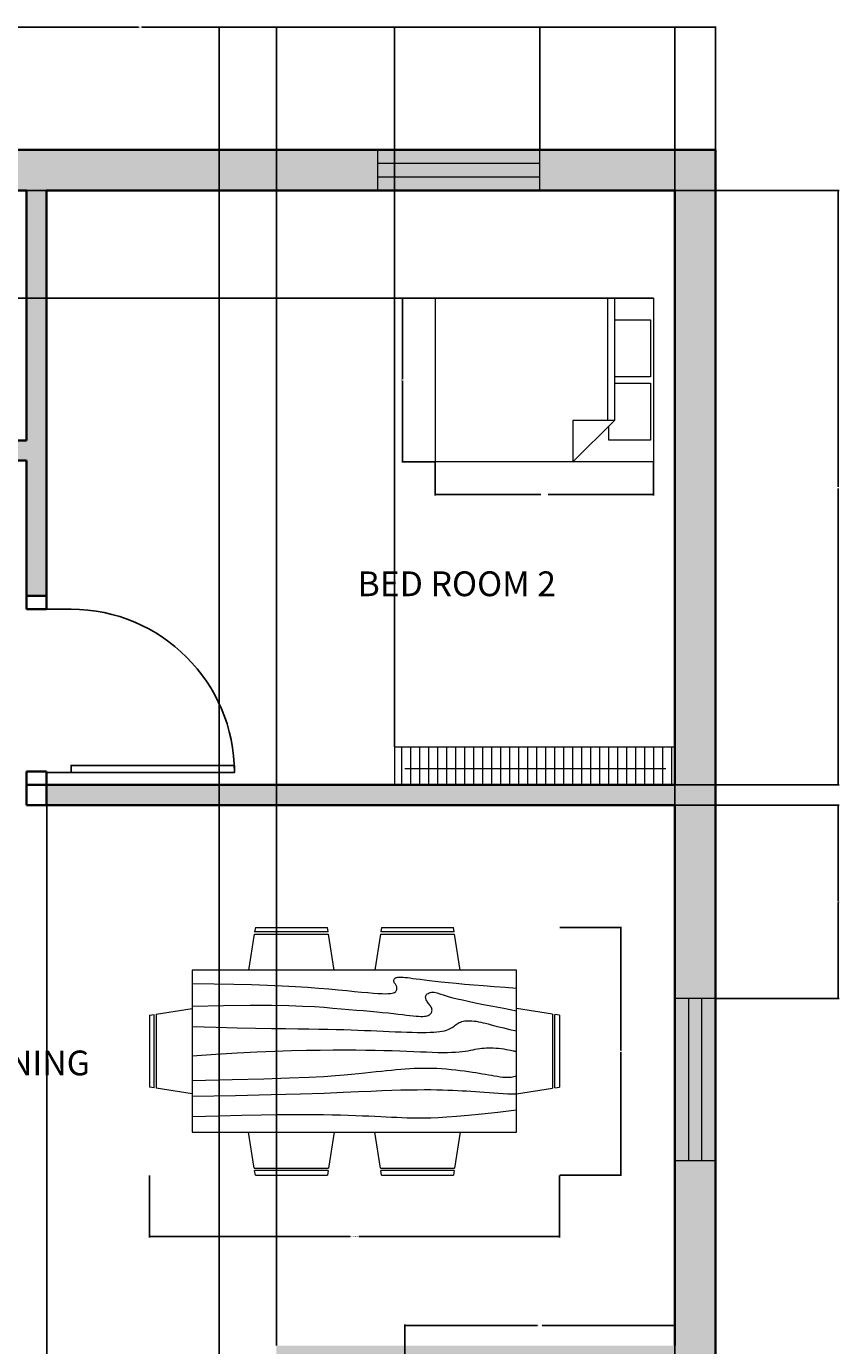
# Model space of a CAD drawing. Units: inches. Extents: x 1839 to 2285, y 722 to 1311.
# Tile 7 of 7: x 2105 to 2285, y 1018 to 1311. Entities that reach past the tile are written whole.
import ezdxf

# ---------------------------------------------------------------- set-up
doc = ezdxf.new("R2010")
doc.units = ezdxf.units.IN
for name, color, linetype, lineweight in [('A-ANNO-DIMS', 2, 'Continuous', 18), ('A-AREA-IDEN', 7, 'Continuous', 18), ('A-DOOR', 3, 'Continuous', 25), ('A-FLOR-CASE', 8, 'Continuous', 18), ('A-FLOR-PATT', 8, 'Continuous', 13), ('A-FURN', 8, 'Continuous', 18), ('A-GLAZ', 4, 'Continuous', 18), ('A-GLAZ-PATT', 9, 'Continuous', 13), ('A-WALL', 7, 'Continuous', 35)]:
    doc.layers.add(name, color=color, linetype=linetype, lineweight=lineweight)
doc.layers.add('A-WALL-PATT', color=18, linetype='Continuous', lineweight=13, true_color=0x000000)
doc.styles.get("Standard").update_dxf_attribs({"font": 'arial.ttf'})
doc.dimstyles.get("Standard").update_dxf_attribs({"dimtxt": 0.18, "dimasz": 0.18, "dimexe": 0.18, "dimexo": 0.0625, "dimgap": 0.09, "dimtad": 0, "dimtih": 1, "dimtoh": 1, "dimdec": 4, "dimzin": 0, "dimdsep": 46, "dimtxsty": 'Standard', "dimcen": 0.09, "dimadec": 0, "dimazin": 0, "dimtfac": 1, "dimtdec": 4, "dimtofl": 0, "dimtmove": 0, "dimatfit": 3, "dimfxl": 1, "dimtolj": 1, "dimtzin": 0, "dimarcsym": 0})

# ---------------------------------------------------------------- blocks, each defined once
blk = doc.blocks.new('*U3')
for p, q in [((0, 0), (0, -6)), ((-40, 0), (-40, -6))]:
    blk.add_line(p, q)
blk.add_lwpolyline([(0, 0), (0, 40), (-1.75, 40), (-1.75, 0)], close=True)
blk.add_arc((0, 0), 40, 90, 180)
blk = doc.blocks.new('Bed - Queen')
for p, q in [((0, -80.00003), (0, 0)), ((0, 0), (59.99999, 0)), ((59.99999, 0), (59.99999, -80.00003)), ((7.99999, -1.2), (28.79998, -1.2)), ((7.99999, -14.4), (7.99999, -1.2)), ((28.79998, -1.2), (28.79998, -14.4)), ((31.19999, -1.2), (51.99999, -1.2)), ((31.19999, -14.4), (31.19999, -1.2)), ((51.99999, -1.2), (51.99999, -16.4)), ((0, -14.4), (44.8, -14.4)), ((59.99999, -29.6), (44.8, -14.4)), ((44.8, -14.4), (44.8, -29.6)), ((44.8, -16.8), (0, -16.8)), ((51.99999, -16.4), (46.79936, -16.4)), ((44.8, -29.6), (59.99999, -29.6)), ((59.99999, -80.00003), (0, -80.00003))]:
    blk.add_line(p, q)
blk = doc.blocks.new('Dining Set - 36 x 72 in.')
for p, q in [((-22, 27.5), (-22.1562, 26.50042)), ((-5.8416, 26.5), (-22.1534, 26.5)), ((-22, 27.5), (-6, 27.5)), ((-5.8437, 26.49966), (-6, 27.5)), ((6, 27.5), (5.8438, 26.50042)), ((22.1584, 26.5), (5.8466, 26.5)), ((6, 27.5), (22, 27.5)), ((22.1563, 26.49966), (22, 27.5)), ((-22.2343, 26.00059), (-23.4847, 17.99762)), ((-22.2304, 26), (-5.7608, 26)), ((-4.5152, 17.99762), (-5.7655, 25.99926)), ((5.7657, 26.00059), (4.5153, 17.99762)), ((5.7696, 26), (22.2392, 26)), ((23.4848, 17.99762), (22.2345, 25.99926)), ((36, 18), (-36, 18)), ((-36, 18), (-36, -18)), ((36, -18), (36, 18)), ((-44.0006, 8.23428), (-35.9976, 9.48474)), ((44.0006, 8.23428), (35.9976, 9.48474)), ((-45.5, 8), (-44.5004, 8.15617)), ((-45.5, 8), (-45.5, -8)), ((-44.5, -8.15843), (-44.5, 8.15338)), ((-44, 8.23041), (-44, -8.23915)), ((44, 8.23041), (44, -8.23915)), ((44.5, -8.15843), (44.5, 8.15338)), ((45.5, 8), (44.5005, 8.15617)), ((45.5, 8), (45.5, -8)), ((-44.4997, -8.15631), (-45.5, -8)), ((-35.9976, -9.48476), (-43.9993, -8.2345)), ((35.9976, -9.48476), (43.9993, -8.2345)), ((44.4997, -8.15631), (45.5, -8)), ((-36, -18), (36, -18)), ((-22.2343, -26.0006), (-23.4847, -17.99762)), ((-4.5152, -17.99762), (-5.7655, -25.99928)), ((5.7657, -26.0006), (4.5153, -17.99762)), ((23.4848, -17.99762), (22.2345, -25.99928)), ((-22.2304, -26), (-5.7608, -26)), ((5.7696, -26), (22.2392, -26)), ((-22, -27.5), (-22.1562, -26.50044)), ((-5.8416, -26.5), (-22.1534, -26.5)), ((-22, -27.5), (-6, -27.5)), ((-5.8437, -26.49967), (-6, -27.5)), ((6, -27.5), (5.8438, -26.50044)), ((22.1584, -26.5), (5.8466, -26.5)), ((6, -27.5), (22, -27.5)), ((22.1563, -26.49967), (22, -27.5))]:
    blk.add_line(p, q)
for points in [[(-36, 15), (-31.1772, 14.97754), (-26.8079, 14.91406), (-22.8538, 14.81543), (-19.276, 14.6875), (-16.0362, 14.53613), (-13.0957, 14.36718), (-10.4159, 14.18652), (-7.9583, 14), (-5.6904, 13.81315), (-3.6035, 13.63021), (-1.6954, 13.45508), (0.0365, 13.29166), (1.5945, 13.14388), (2.9811, 13.01562), (4.1988, 12.9108), (5.25, 12.83333), (6.1393, 12.78613), (6.8802, 12.76823), (7.4883, 12.77767), (7.9792, 12.8125), (8.3685, 12.87077), (8.6719, 12.95052), (8.9049, 13.0498), (9.0833, 13.16666), (9.2205, 13.29899), (9.3216, 13.44401), (9.3895, 13.59879), (9.4271, 13.76041), (9.4373, 13.92594), (9.4232, 14.09245), (9.3875, 14.257), (9.3333, 14.41666), (9.2638, 14.56917), (9.1836, 14.71484), (9.0975, 14.85465), (9.0104, 14.98958), (8.9272, 15.1206), (8.8529, 15.2487), (8.7922, 15.37483), (8.75, 15.5), (8.7305, 15.62467), (8.7344, 15.74739), (8.7617, 15.86621), (8.8125, 15.97916), (8.8867, 16.08431), (8.9844, 16.17968), (9.1055, 16.26334), (9.25, 16.33333), (9.4189, 16.38802), (9.6172, 16.42708), (9.8506, 16.45052), (10.125, 16.45833), (10.4463, 16.45052), (10.8203, 16.42708), (11.2529, 16.38802), (11.75, 16.33333), (12.3184, 16.26318), (12.9694, 16.17838), (13.7151, 16.07991), (14.5677, 15.96875), (15.5395, 15.84586), (16.6426, 15.71224), (17.8893, 15.56884), (19.2917, 15.41666), (20.859, 15.25667), (22.5879, 15.08984), (24.4721, 14.91715), (26.5052, 14.73958), (28.6809, 14.5581), (30.9929, 14.3737), (33.4347, 14.18733), (36, 14)], [(-36, 10), (-28.9766, 10.14274), (-23.1725, 10.20442), (-18.4241, 10.19775), (-14.5677, 10.13541), (-11.4399, 10.03011), (-8.877, 9.89453), (-6.7154, 9.74137), (-4.7917, 9.58333), (-2.9698, 9.43082), (-1.2246, 9.28515), (0.4415, 9.14534), (2.026, 9.01041), (3.5266, 8.87939), (4.9408, 8.7513), (6.266, 8.62516), (7.5, 8.5), (8.6411, 8.37549), (9.6914, 8.2539), (10.6538, 8.13818), (11.5312, 8.03125), (12.3267, 7.93603), (13.043, 7.85547), (13.6831, 7.79248), (14.25, 7.75), (14.7471, 7.7303), (15.1797, 7.73307), (15.5537, 7.75732), (15.875, 7.80208), (16.1494, 7.86637), (16.3828, 7.94922), (16.5811, 8.04964), (16.75, 8.16666), (16.8944, 8.29915), (17.0143, 8.44531), (17.1089, 8.60319), (17.1771, 8.77083), (17.218, 8.94629), (17.2305, 9.1276), (17.2137, 9.31282), (17.1667, 9.5), (17.0895, 9.6875), (16.987, 9.875), (16.8649, 10.0625), (16.7292, 10.25), (16.5856, 10.4375), (16.4401, 10.625), (16.2985, 10.8125), (16.1667, 11), (16.05, 11.18733), (15.9518, 11.3737), (15.8752, 11.5581), (15.8229, 11.73958), (15.798, 11.91715), (15.8034, 12.08984), (15.842, 12.25667), (15.9167, 12.41666), (16.0295, 12.56836), (16.1784, 12.70833), (16.3605, 12.83268), (16.5729, 12.9375), (16.8127, 13.01888), (17.0768, 13.07291), (17.3625, 13.0957), (17.6667, 13.08333), (17.9894, 13.03312), (18.3418, 12.94726), (18.7382, 12.82918), (19.1927, 12.68229), (19.7195, 12.51001), (20.3327, 12.31575), (21.0465, 12.10294), (21.875, 11.875), (22.8357, 11.63354), (23.959, 11.37304), (25.2786, 11.08618), (26.8282, 10.76562), (28.6414, 10.40405), (30.752, 9.99414), (33.1936, 9.52856), (36, 9)], [(-36, 5.5), (-30.7157, 5.3348), (-26.069, 5.20963), (-21.9946, 5.11767), (-18.4271, 5.05208), (-15.3009, 5.00602), (-12.5508, 4.97265), (-10.1112, 4.94515), (-7.9167, 4.91666), (-5.909, 4.88167), (-4.0586, 4.83984), (-2.3429, 4.79215), (-0.7396, 4.73958), (0.7739, 4.6831), (2.22, 4.6237), (3.6213, 4.56233), (5, 4.5), (6.373, 4.43782), (7.7344, 4.3776), (9.0723, 4.32129), (10.375, 4.27083), (11.6309, 4.22819), (12.8281, 4.19531), (13.9551, 4.17415), (15, 4.16666), (15.954, 4.17448), (16.819, 4.19791), (17.6001, 4.23698), (18.3021, 4.29166), (18.9299, 4.36198), (19.4883, 4.44791), (19.9823, 4.54948), (20.4167, 4.66666), (20.7969, 4.79899), (21.1302, 4.94401), (21.4245, 5.09879), (21.6875, 5.26041), (21.9271, 5.42594), (22.1511, 5.59245), (22.3672, 5.757), (22.5834, 5.91666), (22.8065, 6.06868), (23.0404, 6.21093), (23.2879, 6.34147), (23.5521, 6.45833), (23.8358, 6.55957), (24.142, 6.64323), (24.4735, 6.70735), (24.8334, 6.75), (25.2235, 6.76969), (25.642, 6.76692), (26.0858, 6.74267), (26.5521, 6.69791), (27.0379, 6.63362), (27.5404, 6.55078), (28.0565, 6.45036), (28.5834, 6.33333), (29.1242, 6.19987), (29.7071, 6.04687), (30.3661, 5.87044), (31.1354, 5.66666), (32.0493, 5.43164), (33.142, 5.16146), (34.4475, 4.85221), (36, 4.5)], [(-36, -1), (-30.7915, -0.6591), (-26.0195, -0.38216), (-21.6519, -0.16284), (-17.6563, 0.00521), (-14.0005, 0.12833), (-10.6523, 0.21289), (-7.5796, 0.26522), (-4.75, 0.29166), (-2.134, 0.29793), (0.2878, 0.28711), (2.5317, 0.26163), (4.6146, 0.22396), (6.5529, 0.17651), (8.3633, 0.12174), (10.0623, 0.06209), (11.6667, 0), (13.1899, -0.06201), (14.6341, -0.1211), (15.9982, -0.17432), (17.2813, -0.21875), (18.4823, -0.25147), (19.6003, -0.26953), (20.6343, -0.27002), (21.5834, -0.25), (22.4481, -0.20768), (23.2357, -0.14584), (23.9549, -0.06836), (24.6146, 0.02083), (25.2235, 0.11784), (25.7904, 0.21875), (26.3241, 0.31966), (26.8334, 0.41666), (27.3265, 0.50618), (27.8099, 0.58593), (28.2894, 0.65397), (28.7709, 0.70833), (29.2601, 0.74707), (29.763, 0.76823), (30.2855, 0.76985), (30.8334, 0.75), (31.4088, 0.70784), (31.9994, 0.64713), (32.589, 0.57275), (33.1615, 0.48958), (33.7008, 0.4025), (34.1908, 0.3164), (34.6153, 0.23616), (34.9584, 0.16666), (35.2099, 0.11165), (35.3848, 0.07031), (35.504, 0.04069), (35.5886, 0.02083), (35.6594, 0.00879), (35.7377, 0.0026), (35.8442, 0.00032), (36, 0)], [(-36, -6.5), (-27.1843, -6.31267), (-20.084, -6.1263), (-14.469, -5.9419), (-10.1094, -5.76042), (-6.7752, -5.58285), (-4.2363, -5.41016), (-2.2629, -5.24333), (-0.625, -5.08334), (0.8708, -4.93099), (2.2715, -4.78646), (3.5872, -4.64974), (4.8281, -4.52084), (6.0046, -4.39974), (7.127, -4.28646), (8.2053, -4.18099), (9.25, -4.08334), (10.2705, -3.99382), (11.2734, -3.91407), (12.2647, -3.84603), (13.25, -3.79167), (14.2354, -3.75293), (15.2266, -3.73177), (16.2295, -3.73015), (17.25, -3.75), (18.2912, -3.79248), (19.3451, -3.85547), (20.4009, -3.93604), (21.4479, -4.03125), (22.4754, -4.13819), (23.4727, -4.25391), (24.4289, -4.37549), (25.3334, -4.5), (26.1785, -4.62492), (26.9694, -4.74935), (27.7145, -4.87281), (28.4219, -4.99479), (29.1, -5.11483), (29.7572, -5.23242), (30.4016, -5.34709), (31.0417, -5.45834), (31.6837, -5.56437), (32.3262, -5.65821), (32.9658, -5.73153), (33.599, -5.77604), (34.2224, -5.78345), (34.8327, -5.74545), (35.4264, -5.65373), (36, -5.5)], [(-36, -10), (-26.4022, -9.81299), (-18.4675, -9.62891), (-11.9839, -9.45069), (-6.7396, -9.28125), (-2.5226, -9.12354), (0.8789, -8.98047), (3.6769, -8.85498), (6.0833, -8.75), (8.2767, -8.66765), (10.3021, -8.60677), (12.1712, -8.56543), (13.8958, -8.54167), (15.4876, -8.53353), (16.9583, -8.53907), (18.3197, -8.55632), (19.5834, -8.58334), (20.7616, -8.61841), (21.8685, -8.66081), (22.9188, -8.71004), (23.9271, -8.76563), (24.9081, -8.82707), (25.8763, -8.89388), (26.8465, -8.96558), (27.8334, -9.04167), (28.8474, -9.12118), (29.8828, -9.20117), (30.93, -9.27824), (31.9792, -9.34896), (33.0205, -9.40991), (34.0443, -9.45768), (35.0407, -9.48885), (36, -9.5)], [(-36, -14.5), (-30.0881, -14.33513), (-25.0332, -14.21224), (-20.7312, -14.12647), (-17.0781, -14.07292), (-13.97, -14.04671), (-11.3027, -14.04297), (-8.9724, -14.05681), (-6.875, -14.08334), (-4.9224, -14.11833), (-3.0905, -14.16016), (-1.3709, -14.20785), (0.2448, -14.26042), (1.7647, -14.3169), (3.1973, -14.3763), (4.5507, -14.43767), (5.8333, -14.5), (7.0554, -14.5621), (8.235, -14.62175), (9.3922, -14.67652), (10.5469, -14.72396), (11.7192, -14.76164), (12.929, -14.78711), (14.1965, -14.79794), (15.5417, -14.79167), (16.9933, -14.76424), (18.6152, -14.70508), (20.4804, -14.60197), (22.6615, -14.44271), (25.2312, -14.21509), (28.2624, -13.9069), (31.8277, -13.50594), (36, -13)]]:
    blk.add_lwpolyline(points)
blk = doc.blocks.new('WIN-36x9')
for p, q in [((0, 9), (0, 0)), ((36, 9), (0, 9)), ((36, 0), (36, 9)), ((36, 6), (0, 6)), ((0, 3), (36, 3)), ((0, 0), (36, 0))]:
    blk.add_line(p, q)
blk = doc.blocks.new('*D25')
at = {"layer": 'A-ANNO-DIMS', "color": 0, "lineweight": -2, "transparency": 16777216}
for p, q in [((2195.47, 1214.01), (2195.47, 1206.62)), ((2243.94, 1214.01), (2243.94, 1206.62)), ((2195.65, 1206.8), (2218.89, 1206.8)), ((2243.76, 1206.8), (2220.53, 1206.8))]:
    blk.add_line(p, q, dxfattribs=at)
at = {"layer": 'A-ANNO-DIMS', "color": 0, "transparency": 16777216}
for points in [[(2195.65, 1206.83), (2195.65, 1206.77), (2195.47, 1206.8)], [(2243.76, 1206.83), (2243.76, 1206.77), (2243.94, 1206.8)]]:
    blk.add_solid(points, dxfattribs=at)
at = {"layer": 'Defpoints', "color": 0, "transparency": 16777216}
for p in [(2195.47, 1214.07), (2243.94, 1214.07), (2243.94, 1206.8)]:
    blk.add_point(p, dxfattribs=at)
at = {"layer": 'A-ANNO-DIMS', "color": 0, "transparency": 16777216, "insert": (2219.71, 1206.8), "char_height": 0.18, "attachment_point": 5}
blk.add_mtext('\\A1;BED 48 TYP.', dxfattribs=at)
blk = doc.blocks.new('*D26')
at = {"layer": 'A-ANNO-DIMS', "color": 0, "lineweight": -2, "transparency": 16777216}
for p, q in [((2195.41, 1250.42), (2188.02, 1250.42)), ((2188.2, 1250.24), (2188.2, 1232.43)), ((2188.2, 1214.25), (2188.2, 1232.06)), ((2195.41, 1214.07), (2188.02, 1214.07))]:
    blk.add_line(p, q, dxfattribs=at)
at = {"layer": 'A-ANNO-DIMS', "color": 0, "transparency": 16777216}
for points in [[(2188.17, 1250.24), (2188.23, 1250.24), (2188.2, 1250.42)], [(2188.17, 1214.25), (2188.23, 1214.25), (2188.2, 1214.07)]]:
    blk.add_solid(points, dxfattribs=at)
at = {"layer": 'Defpoints', "color": 0, "transparency": 16777216}
for p in [(2195.47, 1250.42), (2188.2, 1214.07), (2195.47, 1214.07)]:
    blk.add_point(p, dxfattribs=at)
at = {"layer": 'A-ANNO-DIMS', "color": 0, "transparency": 16777216, "insert": (2188.2, 1232.25), "char_height": 0.18, "attachment_point": 5}
blk.add_mtext('\\A1;36 TYP.', dxfattribs=at)
blk = doc.blocks.new('*D37')
at = {"layer": 'A-ANNO-DIMS', "color": 0, "lineweight": -2, "transparency": 16777216}
for p, q in [((2188.68, 1013.39), (2188.68, 1022.51)), ((2188.86, 1022.33), (2218.17, 1022.33)), ((2248.5, 1022.33), (2219.18, 1022.33)), ((2248.68, 1013.39), (2248.68, 1022.51))]:
    blk.add_line(p, q, dxfattribs=at)
at = {"layer": 'A-ANNO-DIMS', "color": 0, "transparency": 16777216}
for points in [[(2188.86, 1022.36), (2188.86, 1022.3), (2188.68, 1022.33)], [(2248.5, 1022.36), (2248.5, 1022.3), (2248.68, 1022.33)]]:
    blk.add_solid(points, dxfattribs=at)
at = {"layer": 'Defpoints', "color": 0, "transparency": 16777216}
for p in [(2188.68, 1022.33), (2188.68, 1013.33), (2248.68, 1013.33)]:
    blk.add_point(p, dxfattribs=at)
at = {"layer": 'A-ANNO-DIMS', "color": 0, "transparency": 16777216, "insert": (2218.68, 1022.33), "char_height": 0.18, "attachment_point": 5}
blk.add_mtext('\\A1;TUB 60', dxfattribs=at)
blk = doc.blocks.new('*D39')
at = {"layer": 'A-ANNO-DIMS', "color": 0, "lineweight": -2, "transparency": 16777216}
for p, q in [((2132.01, 1055.64), (2132.01, 1041.87)), ((2223.01, 1055.64), (2223.01, 1041.87)), ((2132.19, 1042.05), (2176.56, 1042.05)), ((2222.83, 1042.05), (2178.46, 1042.05))]:
    blk.add_line(p, q, dxfattribs=at)
at = {"layer": 'A-ANNO-DIMS', "color": 0, "transparency": 16777216}
for points in [[(2132.19, 1042.08), (2132.19, 1042.02), (2132.01, 1042.05)], [(2222.83, 1042.08), (2222.83, 1042.02), (2223.01, 1042.05)]]:
    blk.add_solid(points, dxfattribs=at)
at = {"layer": 'Defpoints', "color": 0, "transparency": 16777216}
for p in [(2132.01, 1055.7), (2223.01, 1055.7), (2223.01, 1042.05)]:
    blk.add_point(p, dxfattribs=at)
at = {"layer": 'A-ANNO-DIMS', "color": 0, "transparency": 16777216, "insert": (2177.51, 1042.05), "char_height": 0.18, "attachment_point": 5}
blk.add_mtext('\\A1;DINING SET 91', dxfattribs=at)
blk = doc.blocks.new('*D40')
at = {"layer": 'A-ANNO-DIMS', "color": 0, "lineweight": -2, "transparency": 16777216}
for p, q in [((2223.08, 1110.7), (2236.84, 1110.7)), ((2236.66, 1110.52), (2236.66, 1083.39)), ((2236.66, 1055.88), (2236.66, 1083.02)), ((2223.08, 1055.7), (2236.84, 1055.7))]:
    blk.add_line(p, q, dxfattribs=at)
at = {"layer": 'A-ANNO-DIMS', "color": 0, "transparency": 16777216}
for points in [[(2236.63, 1110.52), (2236.69, 1110.52), (2236.66, 1110.7)], [(2236.63, 1055.88), (2236.69, 1055.88), (2236.66, 1055.7)]]:
    blk.add_solid(points, dxfattribs=at)
at = {"layer": 'Defpoints', "color": 0, "transparency": 16777216}
for p in [(2223.01, 1110.7), (2236.66, 1110.7), (2223.01, 1055.7)]:
    blk.add_point(p, dxfattribs=at)
at = {"layer": 'A-ANNO-DIMS', "color": 0, "transparency": 16777216, "insert": (2236.66, 1083.2), "char_height": 0.18, "attachment_point": 5}
blk.add_mtext('\\A1;55', dxfattribs=at)
blk = doc.blocks.new('*D45')
at = {"layer": 'A-ANNO-DIMS', "color": 0, "lineweight": -2, "transparency": 16777216}
for p, q in [((2109.18, 1145.02), (2109.18, 722.34)), ((2248.68, 1142.27), (2248.68, 722.34)), ((2109.36, 722.52), (2178.54, 722.52)), ((2248.5, 722.52), (2179.31, 722.52))]:
    blk.add_line(p, q, dxfattribs=at)
at = {"layer": 'A-ANNO-DIMS', "color": 0, "transparency": 16777216}
for points in [[(2109.36, 722.55), (2109.36, 722.49), (2109.18, 722.52)], [(2248.5, 722.55), (2248.5, 722.49), (2248.68, 722.52)]]:
    blk.add_solid(points, dxfattribs=at)
at = {"layer": 'Defpoints', "color": 0, "transparency": 16777216}
for p in [(2109.18, 1145.08), (2248.68, 1142.33), (2248.68, 722.52)]:
    blk.add_point(p, dxfattribs=at)
at = {"layer": 'A-ANNO-DIMS', "color": 0, "transparency": 16777216, "insert": (2178.93, 722.52), "char_height": 0.18, "attachment_point": 5}
blk.add_mtext('\\A1;139.5', dxfattribs=at)
blk = doc.blocks.new('*D46')
at = {"layer": 'A-ANNO-DIMS', "color": 0, "lineweight": -2, "transparency": 16777216}
for p, q in [((2248.74, 1274.33), (2285.11, 1274.33)), ((2284.93, 1274.15), (2284.93, 1208.51)), ((2284.93, 1142.51), (2284.93, 1208.15)), ((2248.74, 1142.33), (2285.11, 1142.33))]:
    blk.add_line(p, q, dxfattribs=at)
at = {"layer": 'A-ANNO-DIMS', "color": 0, "transparency": 16777216}
for points in [[(2284.9, 1274.15), (2284.96, 1274.15), (2284.93, 1274.33)], [(2284.9, 1142.51), (2284.96, 1142.51), (2284.93, 1142.33)]]:
    blk.add_solid(points, dxfattribs=at)
at = {"layer": 'Defpoints', "color": 0, "transparency": 16777216}
for p in [(2248.68, 1274.33), (2284.93, 1274.33), (2248.68, 1142.33)]:
    blk.add_point(p, dxfattribs=at)
at = {"layer": 'A-ANNO-DIMS', "color": 0, "transparency": 16777216, "insert": (2284.93, 1208.33), "char_height": 0.18, "attachment_point": 5}
blk.add_mtext('\\A1;132', dxfattribs=at)
blk = doc.blocks.new('*D53')
at = {"layer": 'A-ANNO-DIMS', "color": 0, "lineweight": -2, "transparency": 16777216}
for p, q in [((2099.66, 1017.89), (2099.66, 1310.76)), ((2099.84, 1310.58), (2129.54, 1310.58)), ((2160, 1310.58), (2130.3, 1310.58)), ((2160.18, 1017.89), (2160.18, 1310.76))]:
    blk.add_line(p, q, dxfattribs=at)
at = {"layer": 'A-ANNO-DIMS', "color": 0, "transparency": 16777216}
for points in [[(2099.84, 1310.61), (2099.84, 1310.55), (2099.66, 1310.58)], [(2160, 1310.61), (2160, 1310.55), (2160.18, 1310.58)]]:
    blk.add_solid(points, dxfattribs=at)
at = {"layer": 'Defpoints', "color": 0, "transparency": 16777216}
for p in [(2160.18, 1310.58), (2099.66, 1017.83), (2160.18, 1017.83)]:
    blk.add_point(p, dxfattribs=at)
at = {"layer": 'A-ANNO-DIMS', "color": 0, "transparency": 16777216, "insert": (2129.92, 1310.58), "char_height": 0.18, "attachment_point": 5}
blk.add_mtext('\\A1;60.51', dxfattribs=at)
blk = doc.blocks.new('*D56')
at = {"layer": 'A-ANNO-DIMS', "color": 0, "lineweight": -2, "transparency": 16777216}
for p, q in [((2147.5, 850.18), (2147.5, 1310.76)), ((2147.68, 1310.58), (2197.64, 1310.58)), ((2248.5, 1310.58), (2198.55, 1310.58)), ((2248.68, 850.18), (2248.68, 1310.76))]:
    blk.add_line(p, q, dxfattribs=at)
at = {"layer": 'A-ANNO-DIMS', "color": 0, "transparency": 16777216}
for points in [[(2147.68, 1310.61), (2147.68, 1310.55), (2147.5, 1310.58)], [(2248.5, 1310.61), (2248.5, 1310.55), (2248.68, 1310.58)]]:
    blk.add_solid(points, dxfattribs=at)
at = {"layer": 'Defpoints', "color": 0, "transparency": 16777216}
for p in [(2248.68, 1310.58), (2147.5, 850.11), (2248.68, 850.11)]:
    blk.add_point(p, dxfattribs=at)
at = {"layer": 'A-ANNO-DIMS', "color": 0, "transparency": 16777216, "insert": (2198.09, 1310.58), "char_height": 0.18, "attachment_point": 5}
blk.add_mtext('\\A1;101.17', dxfattribs=at)
blk = doc.blocks.new('*D61')
at = {"layer": 'A-ANNO-DIMS', "color": 0, "lineweight": -2, "transparency": 16777216}
for p, q in [((2218.64, 1283.39), (2218.64, 1310.76)), ((2218.82, 1310.58), (2237.7, 1310.58)), ((2257.5, 1310.58), (2238.62, 1310.58)), ((2257.68, 1283.39), (2257.68, 1310.76))]:
    blk.add_line(p, q, dxfattribs=at)
at = {"layer": 'A-ANNO-DIMS', "color": 0, "transparency": 16777216}
for points in [[(2218.82, 1310.61), (2218.82, 1310.55), (2218.64, 1310.58)], [(2257.5, 1310.61), (2257.5, 1310.55), (2257.68, 1310.58)]]:
    blk.add_solid(points, dxfattribs=at)
at = {"layer": 'Defpoints', "color": 0, "transparency": 16777216}
for p in [(2257.68, 1310.58), (2218.64, 1283.33), (2257.68, 1283.33)]:
    blk.add_point(p, dxfattribs=at)
at = {"layer": 'A-ANNO-DIMS', "color": 0, "transparency": 16777216, "insert": (2238.16, 1310.58), "char_height": 0.18, "attachment_point": 5}
blk.add_mtext('\\A1;39.036', dxfattribs=at)
blk = doc.blocks.new('*D62')
at = {"layer": 'A-ANNO-DIMS', "color": 0, "lineweight": -2, "transparency": 16777216}
for p, q in [((2248.74, 1137.83), (2285.11, 1137.83)), ((2284.93, 1137.65), (2284.93, 1116.55)), ((2284.93, 1095.09), (2284.93, 1116.19)), ((2257.74, 1094.91), (2285.11, 1094.91))]:
    blk.add_line(p, q, dxfattribs=at)
at = {"layer": 'A-ANNO-DIMS', "color": 0, "transparency": 16777216}
for points in [[(2284.9, 1137.65), (2284.96, 1137.65), (2284.93, 1137.83)], [(2284.9, 1095.09), (2284.96, 1095.09), (2284.93, 1094.91)]]:
    blk.add_solid(points, dxfattribs=at)
at = {"layer": 'Defpoints', "color": 0, "transparency": 16777216}
for p in [(2248.68, 1137.83), (2284.93, 1137.83), (2257.68, 1094.91)]:
    blk.add_point(p, dxfattribs=at)
at = {"layer": 'A-ANNO-DIMS', "color": 0, "transparency": 16777216, "insert": (2284.93, 1116.37), "char_height": 0.18, "attachment_point": 5}
blk.add_mtext('\\A1;42.92', dxfattribs=at)
blk = doc.blocks.new('*D74')
at = {"layer": 'A-ANNO-DIMS', "color": 0, "lineweight": -2, "transparency": 16777216}
for p, q in [((2186.4, 1150.77), (2186.4, 1310.76)), ((2186.58, 1310.58), (2217.14, 1310.58)), ((2248.5, 1310.58), (2217.93, 1310.58)), ((2248.68, 1150.77), (2248.68, 1310.76))]:
    blk.add_line(p, q, dxfattribs=at)
at = {"layer": 'A-ANNO-DIMS', "color": 0, "transparency": 16777216}
for points in [[(2186.58, 1310.61), (2186.58, 1310.55), (2186.4, 1310.58)], [(2248.5, 1310.61), (2248.5, 1310.55), (2248.68, 1310.58)]]:
    blk.add_solid(points, dxfattribs=at)
at = {"layer": 'Defpoints', "color": 0, "transparency": 16777216}
for p in [(2248.68, 1310.58), (2186.4, 1150.7), (2248.68, 1150.7)]:
    blk.add_point(p, dxfattribs=at)
at = {"layer": 'A-ANNO-DIMS', "color": 0, "transparency": 16777216, "insert": (2217.54, 1310.58), "char_height": 0.18, "attachment_point": 5}
blk.add_mtext('\\A1;62.28', dxfattribs=at)
blk = doc.blocks.new('*D78')
at = {"layer": 'A-ANNO-DIMS', "color": 0, "lineweight": -2, "transparency": 16777216}
for p, q in [((2248.61, 1274.33), (1870.25, 1274.33)), ((1870.43, 1274.15), (1870.43, 1262.56)), ((1870.43, 1250.6), (1870.43, 1262.19)), ((2243.88, 1250.42), (1870.25, 1250.42))]:
    blk.add_line(p, q, dxfattribs=at)
at = {"layer": 'A-ANNO-DIMS', "color": 0, "transparency": 16777216}
for points in [[(1870.4, 1274.15), (1870.46, 1274.15), (1870.43, 1274.33)], [(1870.4, 1250.6), (1870.46, 1250.6), (1870.43, 1250.42)]]:
    blk.add_solid(points, dxfattribs=at)
at = {"layer": 'Defpoints', "color": 0, "transparency": 16777216}
for p in [(2248.68, 1274.33), (1870.43, 1250.42), (2243.94, 1250.42)]:
    blk.add_point(p, dxfattribs=at)
at = {"layer": 'A-ANNO-DIMS', "color": 0, "transparency": 16777216, "insert": (1870.43, 1262.38), "char_height": 0.18, "attachment_point": 5}
blk.add_mtext('\\A1;23.91', dxfattribs=at)

msp = doc.modelspace()

# ---------------------------------------------------------------- hatches: boundary and pattern name
at = {"layer": 'A-FLOR-PATT'}
h = msp.add_hatch(dxfattribs=at)
h.set_pattern_fill('ANSI31', color=256, scale=0.629921, angle=45, style=0)
h.paths.add_polyline_path([(2186.4004, 1142.3314), (2248.6771, 1142.3314), (2248.6771, 1150.7042), (2186.4004, 1150.7042)])
at = {"layer": 'A-GLAZ-PATT'}
h = msp.add_hatch(color=256, dxfattribs=at)
h.dxf.hatch_style = 1
h.set_gradient(color1=(0, 0, 255), color2=(255, 255, 0), name='INVCYLINDER')
h.paths.add_polyline_path([(2218.6416, 1283.3314), (2182.6416, 1283.3314), (2182.6416, 1280.3314), (2218.6416, 1280.3314)])
h.paths.add_polyline_path([(2218.6416, 1280.3314), (2182.6416, 1280.3314), (2182.6416, 1277.3314), (2218.6416, 1277.3314)])
h.paths.add_polyline_path([(2218.6416, 1277.3314), (2182.6416, 1277.3314), (2182.6416, 1274.3314), (2218.6416, 1274.3314)])
h = msp.add_hatch(color=256, dxfattribs=at)
h.dxf.hatch_style = 1
h.set_gradient(color1=(0, 0, 255), color2=(255, 255, 0), name='INVCYLINDER')
h.paths.add_polyline_path([(2257.6771, 1094.9086), (2254.6771, 1094.9086), (2254.6771, 1058.9086), (2257.6771, 1058.9086)])
h.paths.add_polyline_path([(2254.6771, 1094.9086), (2251.6771, 1094.9086), (2251.6771, 1058.9086), (2254.6771, 1058.9086)])
h.paths.add_polyline_path([(2251.6771, 1094.9086), (2248.6771, 1094.9086), (2248.6771, 1058.9086), (2251.6771, 1058.9086)])
at = {"layer": 'A-WALL-PATT'}
h = msp.add_hatch(color=256, dxfattribs=at)
h.dxf.hatch_style = 1
h.paths.add_polyline_path([(1906.6771, 1274.3314), (1942.6771, 1274.3314), (1942.6771, 1283.3314), (1897.6771, 1283.3314), (1897.6771, 968.2107), (1906.6771, 968.2107), (1906.6771, 1013.3314), (1939.6771, 1013.3314), (1939.6771, 1017.8314), (1906.6771, 1017.8314), (1906.6771, 1137.8314), (2050.6771, 1137.8314), (2050.6771, 1142.3314), (1906.6771, 1142.3314)])
h.paths.add_polyline_path([(2064.0508, 1283.3314), (1978.6771, 1283.3314), (1978.6771, 1274.3314), (2050.6771, 1274.3314), (2050.6771, 1184.3314), (2055.1771, 1184.3314), (2055.1771, 1214.3314), (2058.1771, 1214.3314), (2058.1771, 1218.8314), (2055.1771, 1218.8314), (2055.1771, 1274.3314), (2064.0508, 1274.3314)])
h.paths.add_polyline_path([(2182.6416, 1283.3314), (2088.0508, 1283.3314), (2088.0508, 1274.3314), (2104.6771, 1274.3314), (2104.6771, 1218.8314), (2094.1771, 1218.8314), (2094.1771, 1214.3314), (2104.6771, 1214.3314), (2104.6771, 1184.3314), (2109.1771, 1184.3314), (2109.1771, 1274.3314), (2182.6416, 1274.3314)])
h.paths.add_polyline_path([(2257.6771, 1283.3314), (2218.6416, 1283.3314), (2218.6416, 1274.3314), (2248.6771, 1274.3314), (2248.6771, 1142.3314), (2186.4004, 1142.3314), (2109.1771, 1142.3314), (2109.1771, 1137.8314), (2248.6771, 1137.8314), (2248.6771, 1094.9086), (2257.6771, 1094.9086)])
h.paths.add_polyline_path([(2257.6771, 1058.9086), (2248.6771, 1058.9086), (2248.6771, 1017.8314), (2160.1771, 1017.8314), (2160.1771, 939.8314), (2164.6771, 939.8314), (2164.6771, 1013.3314), (2248.6771, 1013.3314), (2248.6771, 977.3314), (2248.6771, 950.4862), (2257.6771, 950.4862)])
h.paths.add_polyline_path([(2257.6771, 893.3314), (2248.6771, 893.3314), (2248.6771, 850.1143), (2190.4862, 850.1143), (2190.4862, 845.6143), (2248.6771, 845.6143), (2248.6771, 812.3314), (2100.5038, 812.3314), (2100.5038, 803.3314), (2257.6771, 803.3314)])
h.paths.add_polyline_path([(2257.6771, 926.4862), (2248.6771, 926.4862), (2248.6771, 897.8314), (2141.6642, 897.8314), (2141.6642, 893.3314), (2145.5038, 893.3314), (2145.5038, 812.3314), (2147.5038, 812.3314), (2147.5038, 845.6143), (2153.9854, 845.6143), (2153.9854, 850.1143), (2147.5038, 850.1143), (2147.5038, 893.3314), (2248.6771, 893.3314), (2257.6771, 893.3314)])
h.paths.add_polyline_path([(1906.6771, 893.3314), (1897.6771, 893.3314), (1897.6771, 803.3314), (2022.5038, 803.3314), (2022.5038, 812.3314), (1906.6771, 812.3314)])
h.paths.add_polyline_path([(2031.4676, 897.8314), (1981.6771, 897.8314), (1981.6771, 1013.3314), (2024.6642, 1013.3314), (2024.6642, 1017.8314), (1975.6771, 1017.8314), (1975.6771, 1013.3314), (1978.6771, 1013.3314), (1978.6771, 897.8314), (1906.6771, 897.8314), (1906.6771, 932.2107), (1897.6771, 932.2107), (1897.6771, 893.3314), (1906.6771, 893.3314), (2031.4676, 893.3314)])
h.paths.add_polyline_path([(2099.6642, 1017.8314), (2096.6642, 1017.8314), (2084.1956, 1017.8314), (2084.1956, 1013.3314), (2096.6642, 1013.3314), (2096.6642, 897.8314), (2085.6129, 897.8314), (2085.6129, 893.3314), (2102.6642, 893.3314), (2102.6642, 897.8314), (2099.6642, 897.8314)])

# ---------------------------------------------------------------- linework, layer by layer
at = {"layer": 'A-FLOR-CASE'}
for p, q in [((2248.6771, 1150.7042), (2186.4004, 1150.7042)), ((2186.4004, 1150.7042), (2186.4004, 1142.3314)), ((2248.6771, 1142.3314), (2248.6771, 1150.7042)), ((2188.6771, 1145.9999), (2246.6771, 1145.9999)), ((2186.4004, 1142.3314), (2248.6771, 1142.3314))]:
    msp.add_line(p, q, dxfattribs=at)
at = {"layer": 'A-WALL'}
for p, q in [((2055.1771, 1274.3314), (2104.6771, 1274.3314)), ((2104.6771, 1274.3314), (2104.6771, 1218.8314)), ((2109.1771, 1274.3314), (2109.1771, 1181.3314)), ((2109.1771, 1274.3314), (2248.6771, 1274.3314)), ((2248.6771, 1274.3314), (2248.6771, 1142.3314)), ((2094.1771, 1218.8314), (2104.6771, 1218.8314)), ((2094.1771, 1214.3314), (2104.6771, 1214.3314)), ((2104.6771, 1214.3314), (2104.6771, 1181.3314)), ((2104.6771, 1184.3314), (2109.1771, 1184.3314)), ((2104.6771, 1181.3314), (2109.1771, 1181.3314)), ((2104.6771, 1145.3314), (2109.1771, 1145.3314)), ((2104.6771, 1145.3314), (2104.6771, 1137.8314)), ((2109.1771, 1145.3314), (2109.1771, 1137.8314)), ((2104.6771, 1142.3314), (2248.6771, 1142.3314)), ((2104.6771, 1137.8314), (2248.6771, 1137.8314)), ((2248.6771, 1137.8314), (2248.6771, 1017.8314))]:
    msp.add_line(p, q, dxfattribs=at)
msp.add_lwpolyline([(2022.5038, 803.3314), (1897.6771, 803.3314), (1897.6771, 1283.3314), (2257.6771, 1283.3314), (2257.6771, 803.3314), (2100.5038, 803.3314)], dxfattribs=at)

# ---------------------------------------------------------------- block references
at = {"layer": 'A-DOOR', "xscale": 0.9062393225401889, "yscale": 0.9062393225401889, "zscale": 0.9062393225401889, "rotation": 270}
msp.add_blockref('*U3', (2114.6145, 1145.0819), dxfattribs=at)
at = {"layer": 'A-FURN', "xscale": 0.6058629736700599, "yscale": 0.6058629736700599, "zscale": 0.6058629736700599, "rotation": 270}
msp.add_blockref('Bed - Queen', (2243.9435, 1250.4215), dxfattribs=at)
at = {"layer": 'A-FURN'}
msp.add_blockref('Dining Set - 36 x 72 in.', (2177.5131, 1083.2045), dxfattribs=at)
at = {"layer": 'A-GLAZ'}
msp.add_blockref('WIN-36x9', (2182.642, 1274.331), dxfattribs=at)
at = {"layer": 'A-GLAZ', "rotation": 269.9999999999988}
msp.add_blockref('WIN-36x9', (2248.6767, 1094.9082), dxfattribs=at)

# ---------------------------------------------------------------- texts
at = {"layer": 'A-AREA-IDEN'}
for s, p in [('BED ROOM 2 ', (2178.2022, 1184.2421)), ('LIVING / DINING ', (2063.4967, 1077.8469))]:
    msp.add_text(s, height=5.503795, dxfattribs=at).set_placement(p)

# ---------------------------------------------------------------- dimensions: what is measured, and where the dimension line sits
at = {"layer": 'A-ANNO-DIMS'}
for base, p1, p2, override, picture, middle in [((2160.1771, 1310.5814), (2099.6642, 1017.8314), (2160.1771, 1017.8314), {"dimdec": 2, "dimlfac": 1, "dimrnd": 0, "dimzin": 0, "dimdsep": 46, "dimlunit": 2}, '*D53', (2129.9206, 1310.5814)), ((2248.6771, 1310.5814), (2147.5038, 850.1143), (2248.6771, 850.1143), {"dimdec": 2, "dimlfac": 1, "dimrnd": 0, "dimzin": 0, "dimdsep": 46, "dimlunit": 2}, '*D56', (2198.0905, 1310.5814)), ((2248.6771, 1310.5814), (2186.4004, 1150.7042), (2248.6771, 1150.7042), {"dimdec": 2, "dimlfac": 1, "dimrnd": 0, "dimzin": 0, "dimdsep": 46, "dimlunit": 2}, '*D74', (2217.5388, 1310.5814)), ((2257.67711, 1310.58143), (2218.6416, 1283.33143), (2257.67711, 1283.33143), {"dimdec": 3, "dimlfac": 1, "dimrnd": 0, "dimzin": 0, "dimdsep": 46, "dimlunit": 2}, '*D61', (2238.15935, 1310.58143)), ((2248.6771, 722.516), (2109.1771, 1145.0819), (2248.6771, 1142.3314), {"dimdec": 1, "dimlfac": 1, "dimrnd": 0, "dimzin": 0, "dimdsep": 46, "dimlunit": 2}, '*D45', (2178.9271, 722.516))]:
    dim = msp.add_linear_dim(base=base, p1=p1, p2=p2, dimstyle='Standard', override=override, dxfattribs=at)
    dim.commit()
    dim.dimension.update_dxf_attribs({"geometry": picture, "text_midpoint": middle})
for base, p1, p2, override, picture, middle in [((1870.4271, 1250.4215), (2248.6771, 1274.3314), (2243.9435, 1250.4215), {"dimdec": 2, "dimlfac": 1, "dimrnd": 0, "dimzin": 0, "dimdsep": 46, "dimlunit": 2}, '*D78', (1870.4271, 1262.3765)), ((2284.9271, 1274.3314), (2248.6771, 1142.3314), (2248.6771, 1274.3314), {"dimdec": 0, "dimlfac": 1, "dimrnd": 0, "dimzin": 0, "dimdsep": 46, "dimlunit": 2}, '*D46', (2284.9271, 1208.3314)), ((2284.9271, 1137.8314), (2257.6771, 1094.9086), (2248.6771, 1137.8314), {"dimdec": 2, "dimlfac": 1, "dimrnd": 0, "dimzin": 0, "dimdsep": 46, "dimlunit": 2}, '*D62', (2284.9271, 1116.37)), ((2236.6631, 1110.7045), (2223.0131, 1055.7045), (2223.0131, 1110.7045), {"dimdec": 0, "dimlfac": 1, "dimrnd": 0, "dimzin": 0, "dimdsep": 46, "dimlunit": 2}, '*D40', (2236.6631, 1083.2045))]:
    dim = msp.add_linear_dim(base=base, p1=p1, p2=p2, angle=90, dimstyle='Standard', override=override, dxfattribs=at)
    dim.commit()
    dim.dimension.update_dxf_attribs({"geometry": picture, "text_midpoint": middle})
for base, p1, p2, angle, text, picture, middle in [((2188.2041, 1214.0697), (2195.4745, 1250.4215), (2195.4745, 1214.0697), 270, '<> TYP.', '*D26', (2188.2041, 1232.2456)), ((2188.6771, 1022.3314), (2248.6771, 1013.3314), (2188.6771, 1013.3314), 180, 'TUB <>', '*D37', (2218.6771, 1022.3314))]:
    dim = msp.add_linear_dim(base=base, p1=p1, p2=p2, angle=angle, text=text, dimstyle='Standard', override={"dimdec": 0, "dimlfac": 1, "dimrnd": 0, "dimzin": 0, "dimdsep": 46, "dimlunit": 2}, dxfattribs=at)
    dim.commit()
    dim.dimension.update_dxf_attribs({"geometry": picture, "text_midpoint": middle})
for base, p1, p2, text, picture, middle in [((2243.9435, 1206.7994), (2195.4745, 1214.0697), (2243.9435, 1214.0697), 'BED <> TYP.', '*D25', (2219.709, 1206.7994)), ((2223.0131, 1042.0545), (2132.0131, 1055.7045), (2223.0131, 1055.7045), 'DINING SET <>', '*D39', (2177.5131, 1042.0545))]:
    dim = msp.add_linear_dim(base=base, p1=p1, p2=p2, text=text, dimstyle='Standard', override={"dimdec": 0, "dimlfac": 1, "dimrnd": 0, "dimzin": 0, "dimdsep": 46, "dimlunit": 2}, dxfattribs=at)
    dim.commit()
    dim.dimension.update_dxf_attribs({"geometry": picture, "text_midpoint": middle})

doc.saveas('drawing.dxf')
